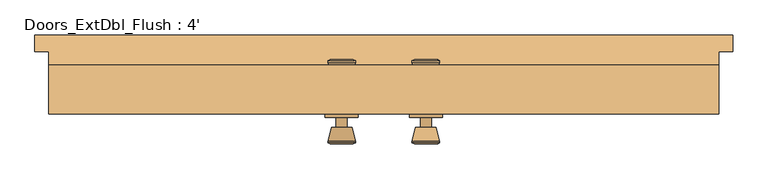
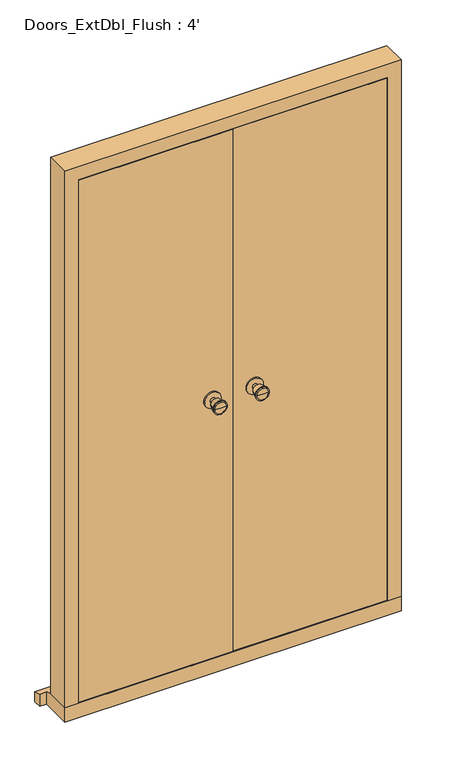
"""IFC4 building model written with IfcOpenShell, lengths in millimetres: door geometry, Doors_ExtDbl_Flush : 4'."""

from ifc_helpers import new_model, si_unit, point, frame, frame_2d, origin, place, context, project, spatial, polyline, circle_curve, trimmed, segment, composite_curve, outline, extrude, faceted_brep, source, transform, mapped, element, save
from ifc_brep_helpers import plane_surface, cylinder_surface, revolved_surface, advanced_brep


def doors_extdbl_flush_4_40db91a8(model_context):
    return source(origin(), model_context, "Body", "SolidModel", [
        advanced_brep(
        [(-76.5, -43.8, 1050.0), (-66.5, -43.8, 1050.0), (-86.5, -43.8, 1050.0), (-96.9758676, -92.8, 1050.0), (-56.0241324, -92.8, 1050.0), (-76.5, -92.8, 1050.0), (-101.5, -90.9721319, 1050.0), (-51.5, -90.9721319, 1050.0), (-101.5, -87.5084537, 1050.0), (-51.5, -87.5084537, 1050.0), (-95.136236, -62.8, 1050.0), (-57.863764, -62.8, 1050.0), (-86.5, -62.8, 1050.0), (-66.5, -62.8, 1050.0)],
        [
            (0, 1),
            (1, 2, circle_curve(frame((-76.5, -43.8, 1050.0), z_axis=(0.0, 1.0, 0.0), x_axis=(1.0, 0.0, 0.0)), 10.0)),
            (2, 0),
            (2, 1, circle_curve(frame((-76.5, -43.8, 1050.0), z_axis=(0.0, 1.0, 0.0), x_axis=(1.0, 0.0, 0.0)), 10.0)),
            (3, 4, circle_curve(frame((-76.5, -92.8, 1050.0), z_axis=(0.0, -1.0, 0.0), x_axis=(1.0, 0.0, 0.0)), 20.4758676)),
            (4, 5),
            (5, 3),
            (4, 3, circle_curve(frame((-76.5, -92.8, 1050.0), z_axis=(0.0, -1.0, 0.0), x_axis=(1.0, 0.0, 0.0)), 20.4758676)),
            (6, 7, circle_curve(frame((-76.5, -90.9721319, 1050.0), z_axis=(0.0, -1.0, 0.0), x_axis=(1.0, 0.0, 0.0)), 25.0)),
            (7, 4),
            (3, 6),
            (7, 6, circle_curve(frame((-76.5, -90.9721319, 1050.0), z_axis=(0.0, -1.0, 0.0), x_axis=(1.0, 0.0, 0.0)), 25.0)),
            (8, 9, circle_curve(frame((-76.5, -87.5084537, 1050.0), z_axis=(0.0, -1.0, 0.0), x_axis=(1.0, 0.0, 0.0)), 25.0)),
            (9, 7),
            (6, 8),
            (9, 8, circle_curve(frame((-76.5, -87.5084537, 1050.0), z_axis=(0.0, -1.0, 0.0), x_axis=(1.0, 0.0, 0.0)), 25.0)),
            (10, 11, circle_curve(frame((-76.5, -62.8, 1050.0), z_axis=(0.0, -1.0, 0.0), x_axis=(1.0, 0.0, 0.0)), 18.636236)),
            (11, 9),
            (8, 10),
            (11, 10, circle_curve(frame((-76.5, -62.8, 1050.0), z_axis=(0.0, -1.0, 0.0), x_axis=(1.0, 0.0, 0.0)), 18.636236)),
            (12, 13, circle_curve(frame((-76.5, -62.8, 1050.0), z_axis=(0.0, -1.0, 0.0), x_axis=(1.0, 0.0, 0.0)), 10.0)),
            (13, 11),
            (10, 12),
            (13, 12, circle_curve(frame((-76.5, -62.8, 1050.0), z_axis=(0.0, -1.0, 0.0), x_axis=(1.0, 0.0, 0.0)), 10.0)),
            (1, 13),
            (12, 2),
        ],
        [
            plane_surface(frame((-76.5, -43.8, 1050.0), z_axis=(0.0, 1.0, 0.0), x_axis=(1.0, 0.0, 0.0))),
            plane_surface(frame((-76.5, -92.8, 1050.0), z_axis=(0.0, -1.0, 0.0), x_axis=(1.0, 0.0, 0.0))),
            revolved_surface(polyline([(-56.0241324, -92.8, 1050.0), (-51.5, -90.9721319, 1050.0)]), (-76.5, -43.8, 1050.0), (0.0, 1.0, 0.0)),
            cylinder_surface(frame((-76.5, -43.8, 1050.0), z_axis=(0.0, 1.0, 0.0), x_axis=(1.0, 0.0, 0.0)), 25.0),
            revolved_surface(polyline([(-51.5, -87.5084537, 1050.0), (-57.863764, -62.8, 1050.0)]), (-76.5, -43.8, 1050.0), (0.0, 1.0, 0.0)),
            plane_surface(frame((-76.5, -62.8, 1050.0), z_axis=(0.0, 1.0, 0.0), x_axis=(1.0, 0.0, 0.0))),
            cylinder_surface(frame((-76.5, -43.8, 1050.0), z_axis=(0.0, 1.0, 0.0), x_axis=(1.0, 0.0, 0.0)), 10.0),
        ],
        [
            (0, [[1, 2, 3]]),
            (0, [[-3, 4, -1]]),
            (1, [[5, 6, 7]]),
            (1, [[8, -7, -6]]),
            (2, [[9, 10, -5, 11]]),
            (2, [[12, -11, -8, -10]]),
            (3, [[13, 14, -9, 15]]),
            (3, [[16, -15, -12, -14]]),
            (4, [[17, 18, -13, 19]]),
            (4, [[20, -19, -16, -18]]),
            (5, [[21, 22, -17, 23]]),
            (5, [[24, -23, -20, -22]]),
            (6, [[-2, 25, -21, 26]]),
            (6, [[-4, -26, -24, -25]]),
        ],
    ),
        extrude(outline(composite_curve([segment(trimmed(circle_curve(frame_2d((1050.0, -76.5)), 30.0), [point((1050.0, -46.5))], [point((1050.0, -106.5))], False, "CARTESIAN"), True, "CONTINUOUS"), segment(trimmed(circle_curve(frame_2d((1050.0, -76.5)), 30.0), [point((1050.0, -106.5))], [point((1050.0, -46.5))], False, "CARTESIAN"), True, "CONTINUOUS")], self_intersect=False)), frame((0.0, -43.8, 0.0), z_axis=(0.0, 1.0, 0.0), x_axis=(0.0, 0.0, 1.0)), (0.0, 0.0, 1.0), 6.0),
        advanced_brep(
        [(-76.5, 12.2, 1050.0), (-86.5, 12.2, 1050.0), (-66.5, 12.2, 1050.0), (-96.9758676, 61.2, 1050.0), (-76.5, 61.2, 1050.0), (-56.0241324, 61.2, 1050.0), (-101.5, 59.3721319, 1050.0), (-51.5, 59.3721319, 1050.0), (-101.5, 55.9084537, 1050.0), (-51.5, 55.9084537, 1050.0), (-95.136236, 31.2, 1050.0), (-57.863764, 31.2, 1050.0), (-86.5, 31.2, 1050.0), (-66.5, 31.2, 1050.0)],
        [
            (0, 1),
            (1, 2, circle_curve(frame((-76.5, 12.2, 1050.0), z_axis=(0.0, -1.0, 0.0), x_axis=(1.0, 0.0, 0.0)), 10.0)),
            (2, 0),
            (2, 1, circle_curve(frame((-76.5, 12.2, 1050.0), z_axis=(0.0, -1.0, 0.0), x_axis=(1.0, 0.0, 0.0)), 10.0)),
            (3, 4),
            (4, 5),
            (5, 3, circle_curve(frame((-76.5, 61.2, 1050.0), z_axis=(0.0, 1.0, 0.0), x_axis=(1.0, 0.0, 0.0)), 20.4758676)),
            (3, 5, circle_curve(frame((-76.5, 61.2, 1050.0), z_axis=(0.0, 1.0, 0.0), x_axis=(1.0, 0.0, 0.0)), 20.4758676)),
            (6, 3),
            (5, 7),
            (7, 6, circle_curve(frame((-76.5, 59.3721319, 1050.0), z_axis=(0.0, 1.0, 0.0), x_axis=(1.0, 0.0, 0.0)), 25.0)),
            (6, 7, circle_curve(frame((-76.5, 59.3721319, 1050.0), z_axis=(0.0, 1.0, 0.0), x_axis=(1.0, 0.0, 0.0)), 25.0)),
            (8, 6),
            (7, 9),
            (9, 8, circle_curve(frame((-76.5, 55.9084537, 1050.0), z_axis=(0.0, 1.0, 0.0), x_axis=(1.0, 0.0, 0.0)), 25.0)),
            (8, 9, circle_curve(frame((-76.5, 55.9084537, 1050.0), z_axis=(0.0, 1.0, 0.0), x_axis=(1.0, 0.0, 0.0)), 25.0)),
            (10, 8),
            (9, 11),
            (11, 10, circle_curve(frame((-76.5, 31.2, 1050.0), z_axis=(0.0, 1.0, 0.0), x_axis=(1.0, 0.0, 0.0)), 18.636236)),
            (10, 11, circle_curve(frame((-76.5, 31.2, 1050.0), z_axis=(0.0, 1.0, 0.0), x_axis=(1.0, 0.0, 0.0)), 18.636236)),
            (12, 10),
            (11, 13),
            (13, 12, circle_curve(frame((-76.5, 31.2, 1050.0), z_axis=(0.0, 1.0, 0.0), x_axis=(1.0, 0.0, 0.0)), 10.0)),
            (12, 13, circle_curve(frame((-76.5, 31.2, 1050.0), z_axis=(0.0, 1.0, 0.0), x_axis=(1.0, 0.0, 0.0)), 10.0)),
            (1, 12),
            (13, 2),
        ],
        [
            plane_surface(frame((-76.5, 12.2, 1050.0), z_axis=(0.0, -1.0, 0.0), x_axis=(1.0, 0.0, 0.0))),
            plane_surface(frame((-76.5, 61.2, 1050.0), z_axis=(0.0, 1.0, 0.0), x_axis=(1.0, 0.0, 0.0))),
            revolved_surface(polyline([(-56.0241324, 61.2, 1050.0), (-51.5, 59.3721319, 1050.0)]), (-76.5, 12.2, 1050.0), (0.0, -1.0, 0.0)),
            cylinder_surface(frame((-76.5, 12.2, 1050.0), z_axis=(0.0, -1.0, 0.0), x_axis=(1.0, 0.0, 0.0)), 25.0),
            revolved_surface(polyline([(-51.5, 55.9084537, 1050.0), (-57.863764, 31.2, 1050.0)]), (-76.5, 12.2, 1050.0), (0.0, -1.0, 0.0)),
            plane_surface(frame((-76.5, 31.2, 1050.0), z_axis=(0.0, -1.0, 0.0), x_axis=(1.0, 0.0, 0.0))),
            cylinder_surface(frame((-76.5, 12.2, 1050.0), z_axis=(0.0, -1.0, 0.0), x_axis=(1.0, 0.0, 0.0)), 10.0),
        ],
        [
            (0, [[1, 2, 3]]),
            (0, [[-3, 4, -1]]),
            (1, [[5, 6, 7]]),
            (1, [[-6, -5, 8]]),
            (2, [[9, -7, 10, 11]]),
            (2, [[-10, -8, -9, 12]]),
            (3, [[13, -11, 14, 15]]),
            (3, [[-14, -12, -13, 16]]),
            (4, [[17, -15, 18, 19]]),
            (4, [[-18, -16, -17, 20]]),
            (5, [[21, -19, 22, 23]]),
            (5, [[-22, -20, -21, 24]]),
            (6, [[25, -23, 26, -2]]),
            (6, [[-26, -24, -25, -4]]),
        ],
    ),
        extrude(outline(composite_curve([segment(trimmed(circle_curve(frame_2d((1050.0, -76.5)), 30.0), [point((1050.0, -46.5))], [point((1050.0, -106.5))], False, "CARTESIAN"), True, "CONTINUOUS"), segment(trimmed(circle_curve(frame_2d((1050.0, -76.5)), 30.0), [point((1050.0, -106.5))], [point((1050.0, -46.5))], False, "CARTESIAN"), True, "CONTINUOUS")], self_intersect=False)), frame((0.0, 6.2, 0.0), z_axis=(0.0, 1.0, 0.0), x_axis=(0.0, 0.0, 1.0)), (0.0, 0.0, 1.0), 6.0),
        advanced_brep(
        [(76.5, -43.8, 1050.0), (86.5, -43.8, 1050.0), (66.5, -43.8, 1050.0), (96.9758676, -92.8, 1050.0), (76.5, -92.8, 1050.0), (56.0241324, -92.8, 1050.0), (101.5, -90.9721319, 1050.0), (51.5, -90.9721319, 1050.0), (101.5, -87.5084537, 1050.0), (51.5, -87.5084537, 1050.0), (95.136236, -62.8, 1050.0), (57.863764, -62.8, 1050.0), (86.5, -62.8, 1050.0), (66.5, -62.8, 1050.0)],
        [
            (0, 1),
            (1, 2, circle_curve(frame((76.5, -43.8, 1050.0), z_axis=(0.0, 1.0, 0.0), x_axis=(-1.0, 0.0, 0.0)), 10.0)),
            (2, 0),
            (2, 1, circle_curve(frame((76.5, -43.8, 1050.0), z_axis=(0.0, 1.0, 0.0), x_axis=(-1.0, 0.0, 0.0)), 10.0)),
            (3, 4),
            (4, 5),
            (5, 3, circle_curve(frame((76.5, -92.8, 1050.0), z_axis=(0.0, -1.0, 0.0), x_axis=(-1.0, 0.0, 0.0)), 20.4758676)),
            (3, 5, circle_curve(frame((76.5, -92.8, 1050.0), z_axis=(0.0, -1.0, 0.0), x_axis=(-1.0, 0.0, 0.0)), 20.4758676)),
            (6, 3),
            (5, 7),
            (7, 6, circle_curve(frame((76.5, -90.9721319, 1050.0), z_axis=(0.0, -1.0, 0.0), x_axis=(-1.0, 0.0, 0.0)), 25.0)),
            (6, 7, circle_curve(frame((76.5, -90.9721319, 1050.0), z_axis=(0.0, -1.0, 0.0), x_axis=(-1.0, 0.0, 0.0)), 25.0)),
            (8, 6),
            (7, 9),
            (9, 8, circle_curve(frame((76.5, -87.5084537, 1050.0), z_axis=(0.0, -1.0, 0.0), x_axis=(-1.0, 0.0, 0.0)), 25.0)),
            (8, 9, circle_curve(frame((76.5, -87.5084537, 1050.0), z_axis=(0.0, -1.0, 0.0), x_axis=(-1.0, 0.0, 0.0)), 25.0)),
            (10, 8),
            (9, 11),
            (11, 10, circle_curve(frame((76.5, -62.8, 1050.0), z_axis=(0.0, -1.0, 0.0), x_axis=(-1.0, 0.0, 0.0)), 18.636236)),
            (10, 11, circle_curve(frame((76.5, -62.8, 1050.0), z_axis=(0.0, -1.0, 0.0), x_axis=(-1.0, 0.0, 0.0)), 18.636236)),
            (12, 10),
            (11, 13),
            (13, 12, circle_curve(frame((76.5, -62.8, 1050.0), z_axis=(0.0, -1.0, 0.0), x_axis=(-1.0, 0.0, 0.0)), 10.0)),
            (12, 13, circle_curve(frame((76.5, -62.8, 1050.0), z_axis=(0.0, -1.0, 0.0), x_axis=(-1.0, 0.0, 0.0)), 10.0)),
            (1, 12),
            (13, 2),
        ],
        [
            plane_surface(frame((76.5, -43.8, 1050.0), z_axis=(0.0, 1.0, 0.0), x_axis=(-1.0, 0.0, 0.0))),
            plane_surface(frame((76.5, -92.8, 1050.0), z_axis=(0.0, -1.0, 0.0), x_axis=(-1.0, 0.0, 0.0))),
            revolved_surface(polyline([(56.0241324, -92.8, 1050.0), (51.5, -90.9721319, 1050.0)]), (76.5, -43.8, 1050.0), (0.0, 1.0, 0.0)),
            cylinder_surface(frame((76.5, -43.8, 1050.0), z_axis=(0.0, 1.0, 0.0), x_axis=(-1.0, 0.0, 0.0)), 25.0),
            revolved_surface(polyline([(51.5, -87.5084537, 1050.0), (57.863764, -62.8, 1050.0)]), (76.5, -43.8, 1050.0), (0.0, 1.0, 0.0)),
            plane_surface(frame((76.5, -62.8, 1050.0), z_axis=(0.0, 1.0, 0.0), x_axis=(-1.0, 0.0, 0.0))),
            cylinder_surface(frame((76.5, -43.8, 1050.0), z_axis=(0.0, 1.0, 0.0), x_axis=(-1.0, 0.0, 0.0)), 10.0),
        ],
        [
            (0, [[1, 2, 3]]),
            (0, [[-3, 4, -1]]),
            (1, [[5, 6, 7]]),
            (1, [[-6, -5, 8]]),
            (2, [[9, -7, 10, 11]]),
            (2, [[-10, -8, -9, 12]]),
            (3, [[13, -11, 14, 15]]),
            (3, [[-14, -12, -13, 16]]),
            (4, [[17, -15, 18, 19]]),
            (4, [[-18, -16, -17, 20]]),
            (5, [[21, -19, 22, 23]]),
            (5, [[-22, -20, -21, 24]]),
            (6, [[25, -23, 26, -2]]),
            (6, [[-26, -24, -25, -4]]),
        ],
    ),
        extrude(outline(composite_curve([segment(trimmed(circle_curve(frame_2d((1050.0, 76.5)), 30.0), [point((1050.0, 46.5))], [point((1050.0, 106.5))], False, "CARTESIAN"), True, "CONTINUOUS"), segment(trimmed(circle_curve(frame_2d((1050.0, 76.5)), 30.0), [point((1050.0, 106.5))], [point((1050.0, 46.5))], False, "CARTESIAN"), True, "CONTINUOUS")], self_intersect=False)), frame((0.0, -43.8, 0.0), z_axis=(0.0, 1.0, 0.0), x_axis=(0.0, 0.0, 1.0)), (0.0, 0.0, 1.0), 6.0),
        advanced_brep(
        [(76.5, 12.2, 1050.0), (66.5, 12.2, 1050.0), (86.5, 12.2, 1050.0), (96.9758676, 61.2, 1050.0), (56.0241324, 61.2, 1050.0), (76.5, 61.2, 1050.0), (101.5, 59.3721319, 1050.0), (51.5, 59.3721319, 1050.0), (101.5, 55.9084537, 1050.0), (51.5, 55.9084537, 1050.0), (95.136236, 31.2, 1050.0), (57.863764, 31.2, 1050.0), (86.5, 31.2, 1050.0), (66.5, 31.2, 1050.0)],
        [
            (0, 1),
            (1, 2, circle_curve(frame((76.5, 12.2, 1050.0), z_axis=(0.0, -1.0, 0.0), x_axis=(-1.0, 0.0, 0.0)), 10.0)),
            (2, 0),
            (2, 1, circle_curve(frame((76.5, 12.2, 1050.0), z_axis=(0.0, -1.0, 0.0), x_axis=(-1.0, 0.0, 0.0)), 10.0)),
            (3, 4, circle_curve(frame((76.5, 61.2, 1050.0), z_axis=(0.0, 1.0, 0.0), x_axis=(-1.0, 0.0, 0.0)), 20.4758676)),
            (4, 5),
            (5, 3),
            (4, 3, circle_curve(frame((76.5, 61.2, 1050.0), z_axis=(0.0, 1.0, 0.0), x_axis=(-1.0, 0.0, 0.0)), 20.4758676)),
            (6, 7, circle_curve(frame((76.5, 59.3721319, 1050.0), z_axis=(0.0, 1.0, 0.0), x_axis=(-1.0, 0.0, 0.0)), 25.0)),
            (7, 4),
            (3, 6),
            (7, 6, circle_curve(frame((76.5, 59.3721319, 1050.0), z_axis=(0.0, 1.0, 0.0), x_axis=(-1.0, 0.0, 0.0)), 25.0)),
            (8, 9, circle_curve(frame((76.5, 55.9084537, 1050.0), z_axis=(0.0, 1.0, 0.0), x_axis=(-1.0, 0.0, 0.0)), 25.0)),
            (9, 7),
            (6, 8),
            (9, 8, circle_curve(frame((76.5, 55.9084537, 1050.0), z_axis=(0.0, 1.0, 0.0), x_axis=(-1.0, 0.0, 0.0)), 25.0)),
            (10, 11, circle_curve(frame((76.5, 31.2, 1050.0), z_axis=(0.0, 1.0, 0.0), x_axis=(-1.0, 0.0, 0.0)), 18.636236)),
            (11, 9),
            (8, 10),
            (11, 10, circle_curve(frame((76.5, 31.2, 1050.0), z_axis=(0.0, 1.0, 0.0), x_axis=(-1.0, 0.0, 0.0)), 18.636236)),
            (12, 13, circle_curve(frame((76.5, 31.2, 1050.0), z_axis=(0.0, 1.0, 0.0), x_axis=(-1.0, 0.0, 0.0)), 10.0)),
            (13, 11),
            (10, 12),
            (13, 12, circle_curve(frame((76.5, 31.2, 1050.0), z_axis=(0.0, 1.0, 0.0), x_axis=(-1.0, 0.0, 0.0)), 10.0)),
            (1, 13),
            (12, 2),
        ],
        [
            plane_surface(frame((76.5, 12.2, 1050.0), z_axis=(0.0, -1.0, 0.0), x_axis=(-1.0, 0.0, 0.0))),
            plane_surface(frame((76.5, 61.2, 1050.0), z_axis=(0.0, 1.0, 0.0), x_axis=(-1.0, 0.0, 0.0))),
            revolved_surface(polyline([(56.0241324, 61.2, 1050.0), (51.5, 59.3721319, 1050.0)]), (76.5, 12.2, 1050.0), (0.0, -1.0, 0.0)),
            cylinder_surface(frame((76.5, 12.2, 1050.0), z_axis=(0.0, -1.0, 0.0), x_axis=(-1.0, 0.0, 0.0)), 25.0),
            revolved_surface(polyline([(51.5, 55.9084537, 1050.0), (57.863764, 31.2, 1050.0)]), (76.5, 12.2, 1050.0), (0.0, -1.0, 0.0)),
            plane_surface(frame((76.5, 31.2, 1050.0), z_axis=(0.0, -1.0, 0.0), x_axis=(-1.0, 0.0, 0.0))),
            cylinder_surface(frame((76.5, 12.2, 1050.0), z_axis=(0.0, -1.0, 0.0), x_axis=(-1.0, 0.0, 0.0)), 10.0),
        ],
        [
            (0, [[1, 2, 3]]),
            (0, [[-3, 4, -1]]),
            (1, [[5, 6, 7]]),
            (1, [[8, -7, -6]]),
            (2, [[9, 10, -5, 11]]),
            (2, [[12, -11, -8, -10]]),
            (3, [[13, 14, -9, 15]]),
            (3, [[16, -15, -12, -14]]),
            (4, [[17, 18, -13, 19]]),
            (4, [[20, -19, -16, -18]]),
            (5, [[21, 22, -17, 23]]),
            (5, [[24, -23, -20, -22]]),
            (6, [[-2, 25, -21, 26]]),
            (6, [[-4, -26, -24, -25]]),
        ],
    ),
        extrude(outline(composite_curve([segment(trimmed(circle_curve(frame_2d((1050.0, 76.5)), 30.0), [point((1050.0, 46.5))], [point((1050.0, 106.5))], False, "CARTESIAN"), True, "CONTINUOUS"), segment(trimmed(circle_curve(frame_2d((1050.0, 76.5)), 30.0), [point((1050.0, 106.5))], [point((1050.0, 46.5))], False, "CARTESIAN"), True, "CONTINUOUS")], self_intersect=False)), frame((0.0, 6.2, 0.0), z_axis=(0.0, 1.0, 0.0), x_axis=(0.0, 0.0, 1.0)), (0.0, 0.0, 1.0), 6.0),
        faceted_brep([(539.1, 51.2, 54.5), (609.6, 51.2, 54.5), (609.6, -37.8, 54.5), (561.1, -37.8, 54.5), (561.1, 9.2, 54.5), (539.1, 9.2, 54.5), (539.1, 51.2, 2039.5), (-539.1, 51.2, 2039.5), (-539.1, 51.2, 54.5), (-609.6, 51.2, 54.5), (-609.6, 51.2, 2110.0), (609.6, 51.2, 2110.0), (609.6, -37.8, 2110.0), (-609.6, -37.8, 2110.0), (-609.6, -37.8, 54.5), (-561.1, -37.8, 54.5), (-561.1, -37.8, 2061.5), (561.1, -37.8, 2061.5), (561.1, 9.2, 2061.5), (-561.1, 9.2, 2061.5), (-561.1, 9.2, 54.5), (-539.1, 9.2, 54.5), (-539.1, 9.2, 2039.5), (539.1, 9.2, 2039.5)], [[[0, 1, 2, 3, 4, 5]], [[1, 0, 6, 7, 8, 9, 10, 11]], [[2, 1, 11, 12]], [[3, 2, 12, 13, 14, 15, 16, 17]], [[4, 3, 17, 18]], [[5, 4, 18, 19, 20, 21, 22, 23]], [[0, 5, 23, 6]], [[7, 22, 21, 8]], [[8, 21, 20, 15, 14, 9]], [[13, 10, 9, 14]], [[19, 16, 15, 20]], [[12, 11, 10, 13]], [[18, 17, 16, 19]], [[6, 23, 22, 7]]]),
        faceted_brep([(634.6, 106.2, 0.0), (634.6, 106.2, 38.5947221), (634.6, 76.2, 47.2703282), (634.6, 76.2, 0.0), (-634.6, 106.2, 38.5947221), (-634.6, 106.2, 0.0), (-634.6, 76.2, 0.0), (-634.6, 76.2, 47.2703282), (609.6, 76.2, 0.0), (609.6, -37.8, 0.0), (-609.6, -37.8, 0.0), (-609.6, 76.2, 0.0), (-609.6, 76.2, 47.2703282), (-609.6, 51.2, 54.5), (609.6, 51.2, 54.5), (609.6, 76.2, 47.2703282), (-609.6, -37.8, 54.5), (609.6, -37.8, 54.5)], [[[0, 1, 2, 3]], [[4, 5, 6, 7]], [[5, 0, 3, 8, 9, 10, 11, 6]], [[1, 0, 5, 4]], [[1, 4, 7, 12, 13, 14, 15, 2]], [[13, 16, 17, 14]], [[16, 10, 9, 17]], [[12, 11, 10, 16, 13]], [[11, 12, 7, 6]], [[8, 15, 14, 17, 9]], [[15, 8, 3, 2]]]),
        extrude(outline(polyline([(558.1, -37.8), (1.5, -37.8), (1.5, 6.2), (558.1, 6.2), (558.1, -37.8)])), frame((0.0, 0.0, 58.5), z_axis=(0.0, 0.0, 1.0), x_axis=(1.0, 0.0, 0.0)), (0.0, 0.0, 1.0), 2000.0),
        extrude(outline(polyline([(-1.5, -37.8), (-558.1, -37.8), (-558.1, 6.2), (-1.5, 6.2), (-1.5, -37.8)])), frame((0.0, 0.0, 58.5), z_axis=(0.0, 0.0, 1.0), x_axis=(1.0, 0.0, 0.0)), (0.0, 0.0, 1.0), 2000.0),
    ])


if __name__ == "__main__":
    model = new_model("IFC4")
    model_context = context("Model", 3, world=origin())
    ifc_project = project(units=[si_unit("LENGTHUNIT", "METRE", prefix="MILLI")], contexts=[model_context])
    site = spatial("IfcSite", under=ifc_project)
    building = spatial("IfcBuilding", under=site)
    placement = place(None, origin())
    doors_extdbl_flush_4_shape = doors_extdbl_flush_4_40db91a8(model_context)
    element("IfcDoor", 1, ObjectType="Doors_ExtDbl_Flush : 4'", at=placement, inside=building, context=model_context, shape_type="MappedRepresentation", body=[
        mapped(doors_extdbl_flush_4_shape, transform((0.0, 0.0, 0.0), x_axis=(1.0, 0.0, 0.0), y_axis=(0.0, 1.0, 0.0), z_axis=(0.0, 0.0, 1.0))),
    ])
    save(model, "model.ifc")

# Revit data of these elements
# Type "Doors_ExtDbl_Flush : 4'"
#   Type Mark = "56"
#   Type Comments = "External Double"
#   Operation = "DoubleDoorSingleSwing"
#   Keynote = "L20"
#   Analytic Construction = "Metal"
#   Wrap Layers (Ext) from Ext = 102.5 mm
#   Wrap Layers (Int) from Ext = 177.5 mm
#   Thickness = 44 mm
#   Rough Width = 1219.2 mm
#   Rough Height = 2110 mm
#   O/A Frame Width = 64 mm
#   Heat Transfer Coefficient (U) = 3.7021 W/(m²·K)
#   Handle Z Distance = 1050 mm
#   FrameWidth = 42 mm
#   FrameOffset - External = 25 mm
#   FrameDepth = 89 mm
#   Door Panel Width = 556.6 mm
#   Door Panel Thickness = 44 mm
#   Door Panel Height = 2000 mm
#   Cill Thickness = 54.5 mm
#   Cill Projection = 30 mm
#   Handle X Distance = 75 mm
#   Height = 2110 mm
#   Structural Tolerance = 6.5 mm
#   Tolerance = 3 mm
#   Undercut = 4 mm
#   Width = 1219.2 mm
#   Cill Extension = 25 mm
#   Cavity Closer Width = 50 mm
#   Cavity Closer Offset from Ext = 102.5 mm
#   Cavity Closer Depth = 85 mm
#   Vis - Ironmongery = yes
#   Vis - Cavity Closers = yes
#   Function = 1
#   Material Door = Door - Panel
#   Material Frame = Door - Frame/Mullion
#   Material Ironmongery = Door - Handle
#   Visual Light Transmittance = 0
#   Thermal Resistance (R) = 0
#   Solar Heat Gain Coefficient = 0
#   Wall Closure = (empty or 0)
# Element 1 (IfcDoor, "Doors_ExtDbl_Flush : 4'")
#   Materials on its faces: "Door - Handle", "Door - Frame/Mullion", "Door - Panel"
# Materials
#   "Door - Panel": class "Wood", colour RGB 210 159 95, transparency 0, Keynote = "L20", Cost = 0
#   "Door - Frame/Mullion": class "Wood", colour RGB 212 179 113, transparency 0, Keynote = "L20", Cost = 0
#   "Door - Handle": colour RGB 0 0 0, transparency 0, Keynote = "P21", Cost = 0
